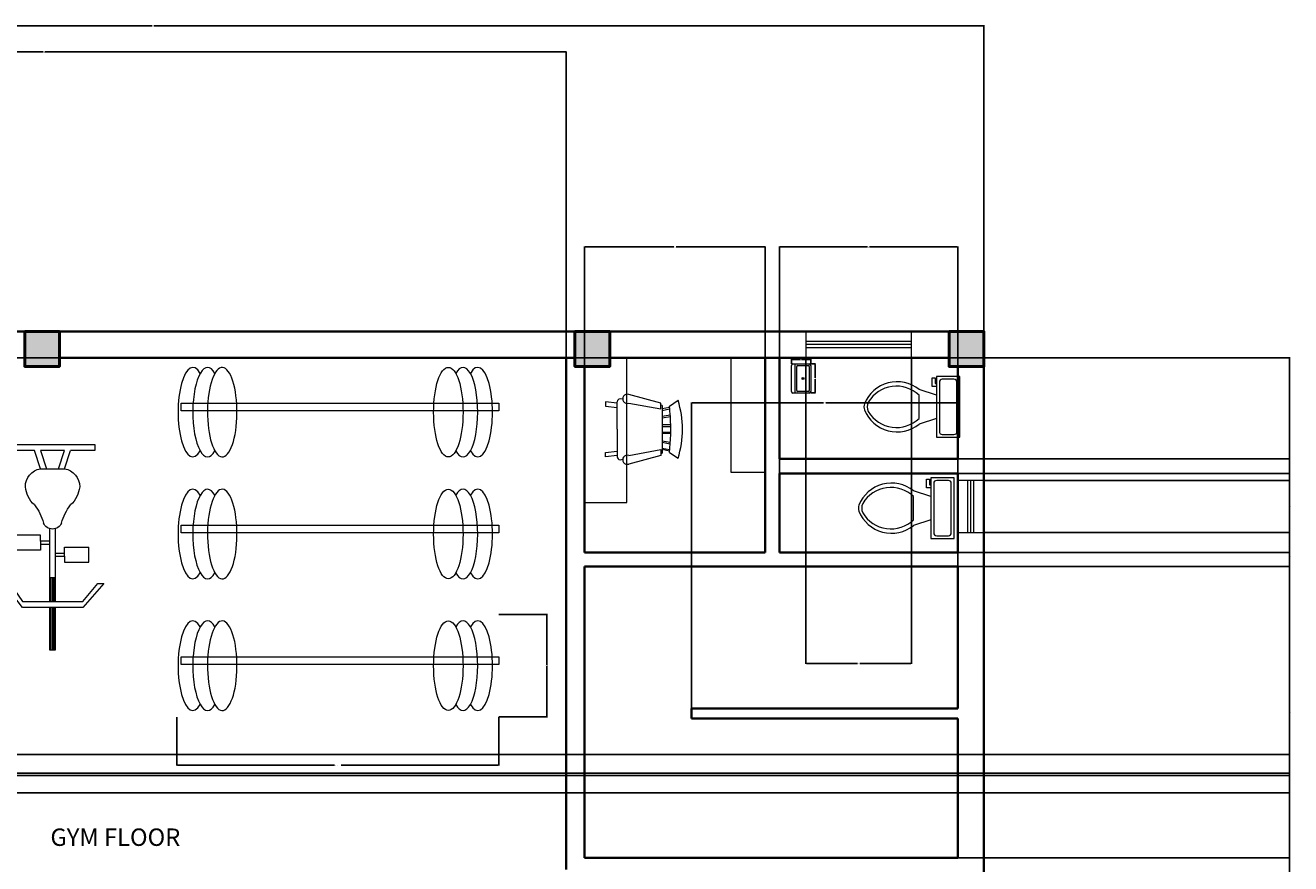
# Model space of a CAD drawing. Units: inches. Extents: x 369 to 4994, y 516 to 1297.
# Tile 9 of 9: x 2235 to 2672, y 855 to 1144. Entities that reach past the tile are written whole.
import ezdxf

# ---------------------------------------------------------------- set-up
doc = ezdxf.new("R2010")
doc.units = ezdxf.units.IN
doc.header["$MEASUREMENT"] = 0
for name, color, linetype, lineweight in [('A-ANNO-DIMS', 2, 'Continuous', 18), ('A-AREA-IDEN', 7, 'Continuous', 18), ('A-COLS', 7, 'Continuous', 50), ('A-EQPM', 9, 'Continuous', 18), ('A-FLOR-CASE', 8, 'Continuous', 18), ('A-FLOR-FIXT', 9, 'Continuous', 18), ('A-FURN', 8, 'Continuous', 18), ('A-GLAZ', 4, 'Continuous', 18), ('A-WALL', 7, 'Continuous', 35)]:
    doc.layers.add(name, color=color, linetype=linetype, lineweight=lineweight)
doc.layers.add('A-COLS-PATT', color=18, linetype='Continuous', lineweight=13, true_color=0x000000)
doc.styles.get("Standard").update_dxf_attribs({"font": 'arial.ttf'})
doc.dimstyles.get("Standard").update_dxf_attribs({"dimtxt": 0.18, "dimasz": 0.18, "dimexe": 0.18, "dimexo": 0.0625, "dimgap": 0.09, "dimtad": 0, "dimtih": 1, "dimtoh": 1, "dimdec": 4, "dimzin": 0, "dimdsep": 46, "dimtxsty": 'Standard', "dimcen": 0.09, "dimadec": 0, "dimazin": 0, "dimtfac": 1, "dimtdec": 4, "dimtofl": 0, "dimtmove": 0, "dimatfit": 3, "dimfxl": 1, "dimtolj": 1, "dimtzin": 0, "dimarcsym": 0})

# ---------------------------------------------------------------- blocks, each defined once
blk = doc.blocks.new('Sink-single - 30 in top')
blk.add_line((-15, -3.999996), (15, -3.999996))
for points in [[(-13.5, 0), (13.5, 0)], [(-15, -18.499996), (-15, -1.5)], [(-13.5, -17.499996), (-13.5, -6.499996)], [(-12.5, -5.499996), (12.5, -5.499996)], [(13.5, -6.499996), (13.5, -17.499996)], [(15, -1.5), (15, -18.499996)], [(13.5, -19.999996), (-13.5, -19.999996)], [(12.5, -18.499996), (-12.5, -18.499996)]]:
    blk.add_lwpolyline(points)
for radius in [1, 0.5]:
    blk.add_circle((0, -11.999996), radius)
for centre, radius, start, end in [((-13.5, -1.5), 1.5, 90, 180), ((-12.5, -6.499996), 1, 90, 180), ((12.5, -6.499996), 1, 0, 90), ((13.5, -1.5), 1.5, 0, 90), ((-13.5, -18.499996), 1.5, 180, 270), ((-12.5, -17.499996), 1, 180, 270), ((12.5, -17.499996), 1, 270, 0), ((13.5, -18.499996), 1.5, 270, 0)]:
    blk.add_arc(centre, radius, start, end)
blk = doc.blocks.new('Chair - Rocking')
for p, q in [((-8, -4.5), (-10, -1.5)), ((-4.5, -7), (-4.96674, -4.19951)), ((-4, -7), (-4.40532, -4.16272)), ((-1.5, -4.05012), (-1.5, -7)), ((-1, -7), (-1, -4.05012)), ((1, -7), (1, -4.04655)), ((1.5, -4.05012), (1.5, -7)), ((4, -7), (4.40187, -4.18694)), ((4.5, -7), (4.96761, -4.19437)), ((8, -4.5), (10, -1.5)), ((-9, -7.5), (-12, -18.49999)), ((-7, -7.5), (-9, -7.5)), ((-9, -18.49999), (-7, -7.5)), ((-8.23428, -6.99939), (-8.3093, -7.47958)), ((-8.23041, -7), (8.23915, -7)), ((-7.5, -4.5), (-7, -7)), ((-6.5, -7), (-7.02225, -4.43)), ((6.5, -7), (7, -4.4057)), ((7.5, -4.5), (7, -7)), ((7, -7.5), (9, -7.5)), ((9, -18.49999), (7, -7.5)), ((8.31071, -7.48854), (8.23449, -7.00073)), ((9, -7.5), (12, -18.49999)), ((-10.36644, -20.64523), (-10.5, -21.49999)), ((10.5, -21.49999), (10.3575, -20.58798)), ((-9, -22.49999), (-9.5, -26.49999)), ((0, -22.49999), (-9.5, -22.49999)), ((-8, -26.49999), (-7.5, -22.49999)), ((0, -22.49999), (9.5, -22.49999)), ((8, -26.49999), (7.5, -22.49999)), ((9, -22.49999), (9.5, -26.49999)), ((-9.5, -26.49999), (-8, -26.49999)), ((9.5, -26.49999), (8, -26.49999))]:
    blk.add_line(p, q)
for centre, radius, start, end in [((0, -34.08333), 34.08333, 72.93847, 107.0615), ((0, -68.25004), 64.25, 93.92211, 97.15267), ((0, -68.25004), 64.25, 82.84733, 93.92211), ((-10.5, -18.99999), 1.58114, 161.5651, 18.43495), ((-9.5, -21.49999), 1, 180, 270), ((10.5, -18.99999), 1.58114, 161.5651, 18.43495), ((9.5, -21.49999), 1, 270, 0)]:
    blk.add_arc(centre, radius, start, end)
blk = doc.blocks.new('Toilet - top')
for p, q in [((9.5, -6), (9.5, -2)), ((-10, -8.5), (-8, -8.5)), ((-10, -9.5), (-10, -8.5)), ((-8, -8.5), (-8, -8)), ((-7, -8), (-7, -9.5)), ((-4, -8), (-6, -14)), ((4, -8), (6, -14)), ((-7, -9.5), (-10, -9.5)), ((4, -14), (-4, -14))]:
    blk.add_line(p, q)
blk.add_lwpolyline([(10.5, -8), (10.5, 0), (-10.5, 0), (-10.5, -8)], close=True)
for points in [[(-9.5, -2), (-9.5, -6)], [(8.5, -1), (-8.5, -1)], [(-8.5, -7), (8.5, -7)]]:
    blk.add_lwpolyline(points)
for centre, radius, start, end in [((-8.62, -1.88), 0.884, 81.8699, 188.1301), ((8.62, -1.88), 0.884, 351.8699, 98.1301), ((-8.62, -6.12), 0.884, 171.8699, 278.1301), ((8.62, -6.12), 0.884, 261.8699, 8.1301), ((3.52, -21.58), 12.17, 141.4691, 247.9714), ((4.2, -21.82), 11.33, 136.3677, 238.9468), ((-3.52, -21.58), 12.17, 292.0284, 38.5307), ((-4.2, -21.82), 11.33, 301.053, 43.6321), ((0, -27.88), 4, 245.7318, 294.2682), ((0, -29), 4, 254.8605, 285.1395)]:
    blk.add_arc(centre, radius, start, end)
blk = doc.blocks.new('Exercise Bike')
for p, q in [((-0.75, 10), (-0.75, 17)), ((-0.75, 17), (0.25, 17)), ((-0.5, 17), (-0.5, 9.9929)), ((-0.25, 10), (-0.25, 17)), ((0, 17), (0, 9.9929)), ((0.25, 17), (0.25, 10)), ((-5.25, 10), (-8.25, 6)), ((-7.25, 6), (-5.25, 9)), ((-0.75, 10), (-5.25, 10)), ((-5.25, 9), (4.75, 9)), ((4.75, 10), (-0.75, 10)), ((-0.75, 5), (-0.75, 9)), ((-0.5, 8.9396), (-0.5, 5)), ((-0.25, 5), (-0.25, 9)), ((0, 8.9396), (0, 5)), ((0.25, 9), (0.25, 5)), ((8.25, 6), (4.75, 10)), ((4.75, 9), (7.25, 6)), ((-8.25, 6), (-7.25, 6)), ((-0.75, -3.0635), (-0.75, 5)), ((-0.75, 5), (0.25, 5)), ((0.25, 5), (0.25, -3.0635)), ((7.25, 6), (8.25, 6)), ((1.75, 2.5), (5.75, 2.5)), ((1.75, 1.5), (1.75, 2.5)), ((5.75, 2.5), (5.75, 0)), ((-6.25, -2), (-6.25, 0.5)), ((-2.25, 0.5), (-6.25, 0.5)), ((-2.25, -0.5), (-2.25, 0.5)), ((0.25, 1.5), (1.75, 1.5)), ((0.25, 1), (1.75, 1)), ((1.75, 1.5), (1.75, 0)), ((1.75, 0), (5.75, 0)), ((-2.25, -2), (-6.25, -2)), ((-2.25, -0.5), (-0.75, -0.5)), ((-2.25, -1), (-2.25, -0.5)), ((-2.25, -1), (-2.25, -2)), ((-0.75, -1), (-2.25, -1)), ((-2.25, -13), (-3.25, -16)), ((-2.25, -16), (-1.25, -13)), ((-2.25, -13), (1.75, -13)), ((0.75, -13), (1.75, -16)), ((1.75, -13), (2.75, -16)), ((-7.25, -16), (-7.25, -17)), ((-4.75, -16), (-7.25, -16)), ((-3.25, -16), (-4.75, -16)), ((1.75, -16), (-2.25, -16)), ((6.75, -16), (2.75, -16)), ((6.75, -17), (6.75, -16)), ((-7.25, -17), (6.75, -17))]:
    blk.add_line(p, q)
for centre, radius, start, end in [((-9.6692, -1.9154), 8.1889, 321.6175, 345.2525), ((-0.25, -4.625), 1.625, 22.61987, 157.3801), ((9.1691, -1.9154), 8.1889, 194.7476, 218.3825), ((0.1685, -10.5843), 4.9531, 133.6443, 173.2256), ((-0.6686, -10.5843), 4.9531, 6.774486, 46.35562), ((-1.7006, -10.0005), 3.0494, 179.9906, 259.6205), ((1.2006, -10.0005), 3.0494, 280.3795, 0.009389)]:
    blk.add_arc(centre, radius, start, end)
blk = doc.blocks.new('GYM-BARBELL')
blk.add_lwpolyline([(1.03, 18.49), (110.54, 18.49), (110.54, 15.84), (1.03, 15.84)], close=True)
for centre, start_param, end_param in [((5.08, 15.44), 5.759587, 9.948377), ((10.16, 15.44), 5.759587, 7.828079), ((15.23, 15.44), 1.544894, 7.828079), ((93.18, 15.44), 3.665191429188082, 9.948376736367669), ((98.25, 15.44), 3.665191, 6.806784), ((103.33, 15.44), 2.617994, 6.806784), ((10.16, 15.44), 7.828079, 9.948377), ((98.25, 15.44), 8.901179, 9.948377)]:
    blk.add_ellipse(centre, major_axis=(0, 15.44), ratio=0.328859, start_param=start_param, end_param=end_param)
blk = doc.blocks.new('*D29')
at = {"layer": 'A-ANNO-DIMS', "color": 0, "lineweight": -2, "transparency": 16777216}
for p, q in [((2506.3, 1027.62), (2507.92, 1027.62)), ((2507.74, 1027.44), (2507.74, 1022.8)), ((2507.74, 1017.79), (2507.74, 1022.43)), ((2506.3, 1017.61), (2507.92, 1017.61))]:
    blk.add_line(p, q, dxfattribs=at)
at = {"layer": 'A-ANNO-DIMS', "color": 0, "transparency": 16777216}
for points in [[(2507.71, 1027.44), (2507.77, 1027.44), (2507.74, 1027.62)], [(2507.71, 1017.79), (2507.77, 1017.79), (2507.74, 1017.61)]]:
    blk.add_solid(points, dxfattribs=at)
at = {"layer": 'Defpoints', "color": 0, "transparency": 16777216}
for p in [(2506.24, 1027.62), (2507.74, 1027.62), (2506.24, 1017.61)]:
    blk.add_point(p, dxfattribs=at)
at = {"layer": 'A-ANNO-DIMS', "color": 0, "transparency": 16777216, "insert": (2507.74, 1022.61), "char_height": 0.18, "attachment_point": 5}
blk.add_mtext('\\A1;SINK 10', dxfattribs=at)
blk = doc.blocks.new('*D30')
at = {"layer": 'A-ANNO-DIMS', "color": 0, "lineweight": -2, "transparency": 16777216}
for p, q in [((2499.56, 1027.69), (2499.56, 1029.31)), ((2499.74, 1029.13), (2502.75, 1029.13)), ((2506.06, 1029.13), (2503.04, 1029.13)), ((2506.24, 1027.69), (2506.24, 1029.31))]:
    blk.add_line(p, q, dxfattribs=at)
at = {"layer": 'A-ANNO-DIMS', "color": 0, "transparency": 16777216}
for points in [[(2499.74, 1029.16), (2499.74, 1029.1), (2499.56, 1029.13)], [(2506.06, 1029.16), (2506.06, 1029.1), (2506.24, 1029.13)]]:
    blk.add_solid(points, dxfattribs=at)
at = {"layer": 'Defpoints', "color": 0, "transparency": 16777216}
for p in [(2499.56, 1029.13), (2499.56, 1027.62), (2506.24, 1027.62)]:
    blk.add_point(p, dxfattribs=at)
at = {"layer": 'A-ANNO-DIMS', "color": 0, "transparency": 16777216, "insert": (2502.9, 1029.13), "char_height": 0.18, "attachment_point": 5}
blk.add_mtext('\\A1;7', dxfattribs=at)
blk = doc.blocks.new('*D35')
at = {"layer": 'A-ANNO-DIMS', "color": 0, "lineweight": -2, "transparency": 16777216}
for p, q in [((2287.71, 905.9), (2287.71, 889.14)), ((2398.64, 905.9), (2398.64, 889.14)), ((2287.89, 889.32), (2341.98, 889.32)), ((2398.46, 889.32), (2344.37, 889.32))]:
    blk.add_line(p, q, dxfattribs=at)
at = {"layer": 'A-ANNO-DIMS', "color": 0, "transparency": 16777216}
for points in [[(2287.89, 889.35), (2287.89, 889.29), (2287.71, 889.32)], [(2398.46, 889.35), (2398.46, 889.29), (2398.64, 889.32)]]:
    blk.add_solid(points, dxfattribs=at)
at = {"layer": 'Defpoints', "color": 0, "transparency": 16777216}
for p in [(2287.71, 905.96), (2398.64, 905.96), (2398.64, 889.32)]:
    blk.add_point(p, dxfattribs=at)
at = {"layer": 'A-ANNO-DIMS', "color": 0, "transparency": 16777216, "insert": (2343.18, 889.32), "char_height": 0.18, "attachment_point": 5}
blk.add_mtext('\\A1;BARBELL 111 TYP.', dxfattribs=at)
blk = doc.blocks.new('*D36')
at = {"layer": 'A-ANNO-DIMS', "color": 0, "lineweight": -2, "transparency": 16777216}
for p, q in [((2398.7, 941.23), (2415.46, 941.23)), ((2415.28, 941.05), (2415.28, 923.78)), ((2415.28, 906.14), (2415.28, 923.41)), ((2398.7, 905.96), (2415.46, 905.96))]:
    blk.add_line(p, q, dxfattribs=at)
at = {"layer": 'A-ANNO-DIMS', "color": 0, "transparency": 16777216}
for points in [[(2415.25, 941.05), (2415.31, 941.05), (2415.28, 941.23)], [(2415.25, 906.14), (2415.31, 906.14), (2415.28, 905.96)]]:
    blk.add_solid(points, dxfattribs=at)
at = {"layer": 'Defpoints', "color": 0, "transparency": 16777216}
for p in [(2398.64, 941.23), (2415.28, 941.23), (2398.64, 905.96)]:
    blk.add_point(p, dxfattribs=at)
at = {"layer": 'A-ANNO-DIMS', "color": 0, "transparency": 16777216, "insert": (2415.28, 923.6), "char_height": 0.18, "attachment_point": 5}
blk.add_mtext('\\A1;35 TYP.', dxfattribs=at)
blk = doc.blocks.new('*D46')
at = {"layer": 'A-ANNO-DIMS', "color": 0, "lineweight": -2, "transparency": 16777216}
for p, q in [((978.32, 1029.79), (2671.51, 1029.79)), ((2671.33, 1029.61), (2671.33, 957.97)), ((2671.33, 885.97), (2671.33, 957.61)), ((1038.32, 885.79), (2671.51, 885.79))]:
    blk.add_line(p, q, dxfattribs=at)
at = {"layer": 'A-ANNO-DIMS', "color": 0, "transparency": 16777216}
for points in [[(2671.3, 1029.61), (2671.36, 1029.61), (2671.33, 1029.79)], [(2671.3, 885.97), (2671.36, 885.97), (2671.33, 885.79)]]:
    blk.add_solid(points, dxfattribs=at)
at = {"layer": 'Defpoints', "color": 0, "transparency": 16777216}
for p in [(978.26, 1029.79), (2671.33, 1029.79), (1038.26, 885.79)]:
    blk.add_point(p, dxfattribs=at)
at = {"layer": 'A-ANNO-DIMS', "color": 0, "transparency": 16777216, "insert": (2671.33, 957.79), "char_height": 0.18, "attachment_point": 5}
blk.add_mtext('\\A1;144', dxfattribs=at)
blk = doc.blocks.new('*D47')
at = {"layer": 'A-ANNO-DIMS', "color": 0, "lineweight": -2, "transparency": 16777216}
for p, q in [((1038.32, 879.79), (2671.51, 879.79)), ((2671.33, 879.61), (2671.33, 837.52)), ((2671.33, 795.07), (2671.33, 837.16)), ((1035.32, 794.89), (2671.51, 794.89))]:
    blk.add_line(p, q, dxfattribs=at)
at = {"layer": 'A-ANNO-DIMS', "color": 0, "transparency": 16777216}
for points in [[(2671.3, 879.61), (2671.36, 879.61), (2671.33, 879.79)], [(2671.3, 795.07), (2671.36, 795.07), (2671.33, 794.89)]]:
    blk.add_solid(points, dxfattribs=at)
at = {"layer": 'Defpoints', "color": 0, "transparency": 16777216}
for p in [(1038.26, 879.79), (2671.33, 879.79), (1035.26, 794.89)]:
    blk.add_point(p, dxfattribs=at)
at = {"layer": 'A-ANNO-DIMS', "color": 0, "transparency": 16777216, "insert": (2671.33, 837.34), "char_height": 0.18, "attachment_point": 5}
blk.add_mtext('\\A1;84.9', dxfattribs=at)
blk = doc.blocks.new('*D79')
at = {"layer": 'A-ANNO-DIMS', "color": 0, "lineweight": -2, "transparency": 16777216}
for p, q in [((1769.44, 1029.79), (2671.51, 1029.79)), ((2671.33, 1029.61), (2671.33, 961.56)), ((2671.33, 893.15), (2671.33, 961.2)), ((1772.44, 892.97), (2671.51, 892.97))]:
    blk.add_line(p, q, dxfattribs=at)
at = {"layer": 'A-ANNO-DIMS', "color": 0, "transparency": 16777216}
for points in [[(2671.3, 1029.61), (2671.36, 1029.61), (2671.33, 1029.79)], [(2671.3, 893.15), (2671.36, 893.15), (2671.33, 892.97)]]:
    blk.add_solid(points, dxfattribs=at)
at = {"layer": 'Defpoints', "color": 0, "transparency": 16777216}
for p in [(1769.37, 1029.79), (2671.33, 1029.79), (1772.37, 892.97)]:
    blk.add_point(p, dxfattribs=at)
at = {"layer": 'A-ANNO-DIMS', "color": 0, "transparency": 16777216, "insert": (2671.33, 961.38), "char_height": 0.18, "attachment_point": 5}
blk.add_mtext('\\A1;136.82', dxfattribs=at)
blk = doc.blocks.new('*D80')
at = {"layer": 'A-ANNO-DIMS', "color": 0, "lineweight": -2, "transparency": 16777216}
for p, q in [((1772.44, 886.6), (2671.51, 886.6)), ((2671.33, 886.42), (2671.33, 847.38)), ((2671.33, 807.97), (2671.33, 847.01)), ((1772.44, 807.79), (2671.51, 807.79))]:
    blk.add_line(p, q, dxfattribs=at)
at = {"layer": 'A-ANNO-DIMS', "color": 0, "transparency": 16777216}
for points in [[(2671.3, 886.42), (2671.36, 886.42), (2671.33, 886.6)], [(2671.3, 807.97), (2671.36, 807.97), (2671.33, 807.79)]]:
    blk.add_solid(points, dxfattribs=at)
at = {"layer": 'Defpoints', "color": 0, "transparency": 16777216}
for p in [(1772.37, 886.6), (2671.33, 886.6), (1772.37, 807.79)]:
    blk.add_point(p, dxfattribs=at)
at = {"layer": 'A-ANNO-DIMS', "color": 0, "transparency": 16777216, "insert": (2671.33, 847.19), "char_height": 0.18, "attachment_point": 5}
blk.add_mtext('\\A1;78.81', dxfattribs=at)
blk = doc.blocks.new('*D97')
at = {"layer": 'A-ANNO-DIMS', "color": 0, "lineweight": -2, "transparency": 16777216}
for p, q in [((1992.93, 1038.85), (1992.93, 1144.37)), ((1993.11, 1144.19), (2279.14, 1144.19)), ((2565.75, 1144.19), (2279.72, 1144.19)), ((2565.93, 1038.85), (2565.93, 1144.37))]:
    blk.add_line(p, q, dxfattribs=at)
at = {"layer": 'A-ANNO-DIMS', "color": 0, "transparency": 16777216}
for points in [[(1993.11, 1144.22), (1993.11, 1144.16), (1992.93, 1144.19)], [(2565.75, 1144.22), (2565.75, 1144.16), (2565.93, 1144.19)]]:
    blk.add_solid(points, dxfattribs=at)
at = {"layer": 'Defpoints', "color": 0, "transparency": 16777216}
for p in [(2565.93, 1144.19), (1992.93, 1038.79), (2565.93, 1038.79)]:
    blk.add_point(p, dxfattribs=at)
at = {"layer": 'A-ANNO-DIMS', "color": 0, "transparency": 16777216, "insert": (2279.43, 1144.19), "char_height": 0.18, "attachment_point": 5}
blk.add_mtext('\\A1;573', dxfattribs=at)
blk = doc.blocks.new('*D99')
at = {"layer": 'A-ANNO-DIMS', "color": 0, "lineweight": -2, "transparency": 16777216}
for p, q in [((2061.93, 1029.85), (2061.93, 1135.37)), ((2062.11, 1135.19), (2241.64, 1135.19)), ((2421.75, 1135.19), (2242.22, 1135.19)), ((2421.93, 1029.85), (2421.93, 1135.37))]:
    blk.add_line(p, q, dxfattribs=at)
at = {"layer": 'A-ANNO-DIMS', "color": 0, "transparency": 16777216}
for points in [[(2062.11, 1135.22), (2062.11, 1135.16), (2061.93, 1135.19)], [(2421.75, 1135.22), (2421.75, 1135.16), (2421.93, 1135.19)]]:
    blk.add_solid(points, dxfattribs=at)
at = {"layer": 'Defpoints', "color": 0, "transparency": 16777216}
for p in [(2421.93, 1135.19), (2061.93, 1029.79), (2421.93, 1029.79)]:
    blk.add_point(p, dxfattribs=at)
at = {"layer": 'A-ANNO-DIMS', "color": 0, "transparency": 16777216, "insert": (2241.93, 1135.19), "char_height": 0.18, "attachment_point": 5}
blk.add_mtext('\\A1;360', dxfattribs=at)
blk = doc.blocks.new('*D100')
at = {"layer": 'A-ANNO-DIMS', "color": 0, "lineweight": -2, "transparency": 16777216}
for p, q in [((2428.28, 962.63), (2428.28, 1068.15)), ((2428.46, 1067.97), (2459.03, 1067.97)), ((2490.38, 1067.97), (2459.82, 1067.97)), ((2490.56, 962.63), (2490.56, 1068.15))]:
    blk.add_line(p, q, dxfattribs=at)
at = {"layer": 'A-ANNO-DIMS', "color": 0, "transparency": 16777216}
for points in [[(2428.46, 1068), (2428.46, 1067.94), (2428.28, 1067.97)], [(2490.38, 1068), (2490.38, 1067.94), (2490.56, 1067.97)]]:
    blk.add_solid(points, dxfattribs=at)
at = {"layer": 'Defpoints', "color": 0, "transparency": 16777216}
for p in [(2490.56, 1067.97), (2428.28, 962.57), (2490.56, 962.57)]:
    blk.add_point(p, dxfattribs=at)
at = {"layer": 'A-ANNO-DIMS', "color": 0, "transparency": 16777216, "insert": (2459.42, 1067.97), "char_height": 0.18, "attachment_point": 5}
blk.add_mtext('\\A1;62.28', dxfattribs=at)
blk = doc.blocks.new('*D101')
at = {"layer": 'A-ANNO-DIMS', "color": 0, "lineweight": -2, "transparency": 16777216}
for p, q in [((2495.43, 962.63), (2495.43, 1068.15)), ((2495.61, 1067.97), (2525.85, 1067.97)), ((2556.75, 1067.97), (2526.5, 1067.97)), ((2556.93, 962.63), (2556.93, 1068.15))]:
    blk.add_line(p, q, dxfattribs=at)
at = {"layer": 'A-ANNO-DIMS', "color": 0, "transparency": 16777216}
for points in [[(2495.61, 1068), (2495.61, 1067.94), (2495.43, 1067.97)], [(2556.75, 1068), (2556.75, 1067.94), (2556.93, 1067.97)]]:
    blk.add_solid(points, dxfattribs=at)
at = {"layer": 'Defpoints', "color": 0, "transparency": 16777216}
for p in [(2556.93, 1067.97), (2495.43, 962.57), (2556.93, 962.57)]:
    blk.add_point(p, dxfattribs=at)
at = {"layer": 'A-ANNO-DIMS', "color": 0, "transparency": 16777216, "insert": (2526.18, 1067.97), "char_height": 0.18, "attachment_point": 5}
blk.add_mtext('\\A1;61.5', dxfattribs=at)
blk = doc.blocks.new('*D102')
at = {"layer": 'A-ANNO-DIMS', "color": 0, "lineweight": -2, "transparency": 16777216}
for p, q in [((2553.99, 1029.79), (2671.51, 1029.79)), ((2671.33, 1029.61), (2671.33, 1012.51)), ((2671.33, 995.06), (2671.33, 1012.15)), ((2556.99, 994.88), (2671.51, 994.88))]:
    blk.add_line(p, q, dxfattribs=at)
at = {"layer": 'A-ANNO-DIMS', "color": 0, "transparency": 16777216}
for points in [[(2671.3, 1029.61), (2671.36, 1029.61), (2671.33, 1029.79)], [(2671.3, 995.06), (2671.36, 995.06), (2671.33, 994.88)]]:
    blk.add_solid(points, dxfattribs=at)
at = {"layer": 'Defpoints', "color": 0, "transparency": 16777216}
for p in [(2553.93, 1029.79), (2671.33, 1029.79), (2556.93, 994.88)]:
    blk.add_point(p, dxfattribs=at)
at = {"layer": 'A-ANNO-DIMS', "color": 0, "transparency": 16777216, "insert": (2671.33, 1012.33), "char_height": 0.18, "attachment_point": 5}
blk.add_mtext('\\A1;34.91', dxfattribs=at)
blk = doc.blocks.new('*D103')
at = {"layer": 'A-ANNO-DIMS', "color": 0, "lineweight": -2, "transparency": 16777216}
for p, q in [((2556.99, 989.85), (2671.51, 989.85)), ((2671.33, 989.67), (2671.33, 976.39)), ((2671.33, 962.75), (2671.33, 976.02)), ((2556.99, 962.57), (2671.51, 962.57))]:
    blk.add_line(p, q, dxfattribs=at)
at = {"layer": 'A-ANNO-DIMS', "color": 0, "transparency": 16777216}
for points in [[(2671.3, 989.67), (2671.36, 989.67), (2671.33, 989.85)], [(2671.3, 962.75), (2671.36, 962.75), (2671.33, 962.57)]]:
    blk.add_solid(points, dxfattribs=at)
at = {"layer": 'Defpoints', "color": 0, "transparency": 16777216}
for p in [(2556.93, 989.85), (2671.33, 989.85), (2556.93, 962.57)]:
    blk.add_point(p, dxfattribs=at)
at = {"layer": 'A-ANNO-DIMS', "color": 0, "transparency": 16777216, "insert": (2671.33, 976.21), "char_height": 0.18, "attachment_point": 5}
blk.add_mtext('\\A1;27.28', dxfattribs=at)
blk = doc.blocks.new('*D104')
at = {"layer": 'A-ANNO-DIMS', "color": 0, "lineweight": -2, "transparency": 16777216}
for p, q in [((2556.99, 957.85), (2671.51, 957.85)), ((2671.33, 957.67), (2671.33, 907.78)), ((2671.33, 857.52), (2671.33, 907.41)), ((2556.99, 857.34), (2671.51, 857.34))]:
    blk.add_line(p, q, dxfattribs=at)
at = {"layer": 'A-ANNO-DIMS', "color": 0, "transparency": 16777216}
for points in [[(2671.3, 957.67), (2671.36, 957.67), (2671.33, 957.85)], [(2671.3, 857.52), (2671.36, 857.52), (2671.33, 857.34)]]:
    blk.add_solid(points, dxfattribs=at)
at = {"layer": 'Defpoints', "color": 0, "transparency": 16777216}
for p in [(2556.93, 957.85), (2671.33, 957.85), (2556.93, 857.34)]:
    blk.add_point(p, dxfattribs=at)
at = {"layer": 'A-ANNO-DIMS', "color": 0, "transparency": 16777216, "insert": (2671.33, 907.6), "char_height": 0.18, "attachment_point": 5}
blk.add_mtext('\\A1;100.51', dxfattribs=at)
blk = doc.blocks.new('*D116')
at = {"layer": 'A-ANNO-DIMS', "color": 0, "lineweight": -2, "transparency": 16777216}
for p, q in [((2504.55, 1029.73), (2504.55, 924.21)), ((2540.94, 1029.73), (2540.94, 924.21)), ((2504.73, 924.39), (2522.35, 924.39)), ((2540.76, 924.39), (2523.14, 924.39))]:
    blk.add_line(p, q, dxfattribs=at)
at = {"layer": 'A-ANNO-DIMS', "color": 0, "transparency": 16777216}
for points in [[(2504.73, 924.42), (2504.73, 924.36), (2504.55, 924.39)], [(2540.76, 924.42), (2540.76, 924.36), (2540.94, 924.39)]]:
    blk.add_solid(points, dxfattribs=at)
at = {"layer": 'Defpoints', "color": 0, "transparency": 16777216}
for p in [(2504.55, 1029.79), (2540.94, 1029.79), (2504.55, 924.39)]:
    blk.add_point(p, dxfattribs=at)
at = {"layer": 'A-ANNO-DIMS', "color": 0, "transparency": 16777216, "insert": (2522.75, 924.39), "char_height": 0.18, "attachment_point": 5}
blk.add_mtext('\\A1;36.39', dxfattribs=at)
blk = doc.blocks.new('*D117')
at = {"layer": 'A-ANNO-DIMS', "color": 0, "lineweight": -2, "transparency": 16777216}
for p, q in [((2565.99, 987.42), (2671.51, 987.42)), ((2671.33, 987.24), (2671.33, 978.63)), ((2671.33, 969.66), (2671.33, 978.27)), ((2565.99, 969.48), (2671.51, 969.48))]:
    blk.add_line(p, q, dxfattribs=at)
at = {"layer": 'A-ANNO-DIMS', "color": 0, "transparency": 16777216}
for points in [[(2671.3, 987.24), (2671.36, 987.24), (2671.33, 987.42)], [(2671.3, 969.66), (2671.36, 969.66), (2671.33, 969.48)]]:
    blk.add_solid(points, dxfattribs=at)
at = {"layer": 'Defpoints', "color": 0, "transparency": 16777216}
for p in [(2565.93, 987.42), (2565.93, 969.48), (2671.33, 969.48)]:
    blk.add_point(p, dxfattribs=at)
at = {"layer": 'A-ANNO-DIMS', "color": 0, "transparency": 16777216, "insert": (2671.33, 978.45), "char_height": 0.18, "attachment_point": 5}
blk.add_mtext('\\A1;17.933', dxfattribs=at)
blk = doc.blocks.new('*D120')
at = {"layer": 'A-ANNO-DIMS', "color": 0, "lineweight": -2, "transparency": 16777216}
for p, q in [((2465.17, 908.87), (2465.17, 1014.39)), ((2465.35, 1014.21), (2510.65, 1014.21)), ((2556.75, 1014.21), (2511.44, 1014.21)), ((2556.93, 908.87), (2556.93, 1014.39))]:
    blk.add_line(p, q, dxfattribs=at)
at = {"layer": 'A-ANNO-DIMS', "color": 0, "transparency": 16777216}
for points in [[(2465.35, 1014.24), (2465.35, 1014.18), (2465.17, 1014.21)], [(2556.75, 1014.24), (2556.75, 1014.18), (2556.93, 1014.21)]]:
    blk.add_solid(points, dxfattribs=at)
at = {"layer": 'Defpoints', "color": 0, "transparency": 16777216}
for p in [(2556.93, 1014.21), (2465.17, 908.81), (2556.93, 908.81)]:
    blk.add_point(p, dxfattribs=at)
at = {"layer": 'A-ANNO-DIMS', "color": 0, "transparency": 16777216, "insert": (2511.05, 1014.21), "char_height": 0.18, "attachment_point": 5}
blk.add_mtext('\\A1;91.76', dxfattribs=at)

msp = doc.modelspace()

# ---------------------------------------------------------------- hatches: boundary and pattern name
at = {"layer": 'A-COLS-PATT'}
h = msp.add_hatch(color=256, dxfattribs=at)
h.dxf.hatch_style = 1
h.paths.add_polyline_path([(540.2581, 633.7894), (528.2581, 633.7894), (528.2581, 621.7894), (540.2581, 621.7894)])
h.paths.add_polyline_path([(726.2581, 633.7894), (714.2581, 633.7894), (714.2581, 621.7894), (726.2581, 621.7894)])
h.paths.add_polyline_path([(918.2581, 633.7894), (906.2581, 633.7894), (906.2581, 621.7894), (918.2581, 621.7894)])
h.paths.add_polyline_path([(1047.2581, 633.7894), (1035.2581, 633.7894), (1035.2581, 621.7894), (1047.2581, 621.7894)])
h.paths.add_polyline_path([(1047.2581, 798.6977), (1035.2581, 798.6977), (1035.2581, 786.6977), (1047.2581, 786.6977)])
h.paths.add_polyline_path([(918.2581, 795.7894), (906.2581, 795.7894), (906.2581, 783.7894), (918.2581, 783.7894)])
h.paths.add_polyline_path([(726.2581, 795.7894), (714.2581, 795.7894), (714.2581, 783.7894), (726.2581, 783.7894)])
h.paths.add_polyline_path([(1047.2581, 1038.7894), (1035.2581, 1038.7894), (1035.2581, 1026.7894), (1047.2581, 1026.7894)])
h.paths.add_polyline_path([(855.044, 1038.7894), (843.044, 1038.7894), (843.044, 1026.7894), (855.044, 1026.7894)])
h.paths.add_polyline_path([(728.5536, 1038.7894), (716.5536, 1038.7894), (716.5536, 1026.7894), (728.5536, 1026.7894)])
h.paths.add_polyline_path([(543.2581, 1038.7894), (531.2581, 1038.7894), (531.2581, 1026.7894), (543.2581, 1026.7894)])
h.paths.add_polyline_path([(543.2581, 792.9013), (531.2581, 792.9013), (531.2581, 780.9013), (543.2581, 780.9013), (543.2581, 783.7894)])
h.paths.add_polyline_path([(1274.3738, 633.7894), (1262.3738, 633.7894), (1262.3738, 621.7894), (1274.3738, 621.7894)])
h.paths.add_polyline_path([(1460.3738, 633.7894), (1448.3738, 633.7894), (1448.3738, 621.7894), (1460.3738, 621.7894)])
h.paths.add_polyline_path([(1652.3738, 633.7894), (1640.3738, 633.7894), (1640.3738, 621.7894), (1652.3738, 621.7894)])
h.paths.add_polyline_path([(1781.3738, 633.7894), (1769.3738, 633.7894), (1769.3738, 621.7894), (1781.3738, 621.7894)])
h.paths.add_polyline_path([(1781.3738, 1038.7894), (1769.3738, 1038.7894), (1769.3738, 1026.7894), (1781.3738, 1026.7894)])
h.paths.add_polyline_path([(1625.484, 1038.7894), (1613.484, 1038.7894), (1613.484, 1026.7894), (1615.6962, 1026.7894), (1625.484, 1026.7894)])
h.paths.add_polyline_path([(1462.6692, 1038.7894), (1450.6692, 1038.7894), (1450.6692, 1026.7894), (1462.6692, 1026.7894)])
h.paths.add_polyline_path([(1277.3738, 1038.7894), (1265.3738, 1038.7894), (1265.3738, 1026.7894), (1277.3738, 1026.7894)])
h.paths.add_polyline_path([(1460.3738, 807.7894), (1448.3738, 807.7894), (1448.3738, 795.7894), (1460.3738, 795.7894)])
h.paths.add_polyline_path([(1652.3738, 807.7894), (1640.3738, 807.7894), (1640.3738, 795.7894), (1652.3738, 795.7894)])
h.paths.add_polyline_path([(2244.9265, 633.7894), (2232.9265, 633.7894), (2232.9265, 621.7894), (2244.9265, 621.7894)])
h.paths.add_polyline_path([(2058.9265, 633.7894), (2046.9265, 633.7894), (2046.9265, 621.7894), (2058.9265, 621.7894)])
h.paths.add_polyline_path([(2436.9265, 633.7894), (2424.9265, 633.7894), (2424.9265, 621.7894), (2436.9265, 621.7894)])
h.paths.add_polyline_path([(2565.9265, 633.7894), (2553.9265, 633.7894), (2553.9265, 621.7894), (2565.9265, 621.7894)])
h.paths.add_polyline_path([(2565.9265, 798.6977), (2553.9265, 798.6977), (2553.9265, 786.6977), (2565.9265, 786.6977)])
h.paths.add_polyline_path([(2565.9265, 1038.7894), (2553.9265, 1038.7894), (2553.9265, 1026.7894), (2565.9265, 1026.7894)])
h.paths.add_polyline_path([(2436.9265, 1038.7894), (2424.9265, 1038.7894), (2424.9265, 1026.7894), (2436.9265, 1026.7894)])
h.paths.add_polyline_path([(2247.222, 1038.7894), (2235.222, 1038.7894), (2235.222, 1026.7894), (2247.222, 1026.7894)])
h.paths.add_polyline_path([(2061.9265, 1038.7894), (2049.9265, 1038.7894), (2049.9265, 1026.7894), (2061.9265, 1026.7894)])

# ---------------------------------------------------------------- linework, layer by layer
at = {"layer": 'A-COLS'}
for points in [[(2235.222, 1038.7894), (2247.222, 1038.7894), (2247.222, 1026.7894), (2235.222, 1026.7894)], [(2424.9265, 1038.7894), (2436.9265, 1038.7894), (2436.9265, 1026.7894), (2424.9265, 1026.7894)], [(2553.9265, 1038.7894), (2565.9265, 1038.7894), (2565.9265, 1026.7894), (2553.9265, 1026.7894)]]:
    msp.add_lwpolyline(points, close=True, dxfattribs=at)
at = {"layer": 'A-FLOR-CASE'}
msp.add_lwpolyline([(2428.2834, 1026.7894), (2428.2834, 979.9068), (2442.8807, 979.9068), (2442.8807, 1029.7894), (2436.9265, 1029.7894)], dxfattribs=at)
msp.add_lwpolyline([(2490.5616, 1029.7894), (2478.6323, 1029.7894), (2478.6323, 990.3401), (2490.5616, 990.3401)], close=True, dxfattribs=at)
at = {"layer": 'A-GLAZ'}
for p, q in [((2540.941, 1035.3655), (2504.5526, 1035.3655)), ((2540.941, 1034.2894), (2504.5526, 1034.2894)), ((2540.941, 1033.2133), (2504.5526, 1033.2133)), ((2560.3504, 969.4831), (2560.3504, 987.4162)), ((2561.4265, 969.4831), (2561.4265, 987.4162)), ((2562.5026, 969.4831), (2562.5026, 987.4162))]:
    msp.add_line(p, q, dxfattribs=at)
for points in [[(2504.5526, 1029.7894), (2540.941, 1029.7894), (2540.941, 1038.7894), (2504.5526, 1038.7894)], [(2556.9265, 969.4831), (2565.9265, 969.4831), (2565.9265, 987.4162), (2556.9265, 987.4162)]]:
    msp.add_lwpolyline(points, close=True, dxfattribs=at)
at = {"layer": 'A-WALL'}
for p, q in [((2556.9265, 1038.7894), (2049.9265, 1038.7894)), ((2361.7124, 1029.7894), (2247.222, 1029.7894)), ((2424.9265, 1029.7894), (2247.222, 1029.7894)), ((2424.9265, 1029.7894), (2373.7124, 1029.7894)), ((2421.9265, 908.8078), (2421.9265, 1029.7894)), ((2553.9265, 1029.7894), (2436.9265, 1029.7894)), ((2490.9265, 1029.7894), (2436.9265, 1029.7894)), ((2565.9265, 621.7894), (2565.9265, 1029.7894)), ((2428.2834, 962.568), (2428.2834, 1026.7894)), ((2556.9265, 994.8764), (2556.9265, 1026.7894)), ((2556.9265, 962.568), (2556.9265, 989.8457)), ((2428.2834, 857.3402), (2428.2834, 957.8515)), ((2556.9265, 908.8078), (2556.9265, 957.8515)), ((2421.9265, 908.8078), (2421.9265, 853.3402)), ((2556.9265, 908.8078), (2465.1694, 908.8078)), ((2465.1694, 905.3798), (2465.1694, 908.8078)), ((2556.9265, 905.3798), (2465.1694, 905.3798)), ((2556.9265, 857.3402), (2556.9265, 905.3798)), ((2556.9265, 857.3402), (2556.9265, 879.7894)), ((2556.9265, 857.3402), (2428.2834, 857.3402))]:
    msp.add_line(p, q, dxfattribs=at)
for points in [[(2495.4265, 994.8764), (2495.4265, 1029.7894), (2490.5616, 1029.7894), (2490.5616, 962.568)], [(2490.5616, 994.8764), (2490.5616, 989.8457)], [(2556.9265, 994.8764), (2495.4265, 994.8764)], [(2495.4265, 962.568), (2495.4265, 989.8457)], [(2495.4265, 989.8457), (2556.9265, 989.8457)], [(2490.5616, 962.568), (2428.2834, 962.568)], [(2556.9265, 962.568), (2495.4265, 962.568)], [(2428.2834, 957.8515), (2483.9184, 957.8515)], [(2428.2834, 957.8515), (2556.9265, 957.8515)]]:
    msp.add_lwpolyline(points, dxfattribs=at)

# ---------------------------------------------------------------- block references
at = {"layer": 'A-EQPM'}
for p in [(2288.107, 995.5724), (2288.107, 953.5332), (2288.107, 908.154)]:
    msp.add_blockref('GYM-BARBELL', p, dxfattribs=at)
at = {"layer": 'A-EQPM', "xscale": -2.080401215836593, "yscale": 2.080401215836593, "zscale": 2.080401215836593, "rotation": 180}
msp.add_blockref('Exercise Bike', (2245.3378, 964.4622), dxfattribs=at)
at = {"layer": 'A-FLOR-FIXT', "xscale": 0.3338934755196378, "yscale": 0.3338934755196378, "zscale": 0.3338934755196378, "rotation": 89.99999999999994}
msp.add_blockref('Sink-single - 30 in top', (2499.5577, 1022.6146), dxfattribs=at)
at = {"layer": 'A-FLOR-FIXT', "rotation": 269.9999999999999}
for p in [(2557.5878, 1012.8341), (2555.6766, 977.9149)]:
    msp.add_blockref('Toilet - top', p, dxfattribs=at)
at = {"layer": 'A-FURN', "rotation": 269.999999999998}
msp.add_blockref('Chair - Rocking', (2461.9903, 1005.1034), dxfattribs=at)

# ---------------------------------------------------------------- texts
at = {"layer": 'A-AREA-IDEN'}
msp.add_text(' GYM FLOOR ', height=6, dxfattribs=at).set_placement((2242.2655, 861.4773))

# ---------------------------------------------------------------- dimensions: what is measured, and where the dimension line sits
at = {"layer": 'A-ANNO-DIMS'}
for base, p1, p2, override, picture, middle in [((2565.9265, 1144.1894), (1992.9265, 1038.7894), (2565.9265, 1038.7894), {"dimdec": 0, "dimlfac": 1, "dimrnd": 0, "dimzin": 0, "dimdsep": 46, "dimlunit": 2}, '*D97', (2279.4265, 1144.1894)), ((2421.9265, 1135.1894), (2061.9265, 1029.7894), (2421.9265, 1029.7894), {"dimdec": 0, "dimlfac": 1, "dimrnd": 0, "dimzin": 0, "dimdsep": 46, "dimlunit": 2}, '*D99', (2241.9265, 1135.1894)), ((2490.5616, 1067.968), (2428.2834, 962.568), (2490.5616, 962.568), {"dimdec": 2, "dimlfac": 1, "dimrnd": 0, "dimzin": 0, "dimdsep": 46, "dimlunit": 2}, '*D100', (2459.4225, 1067.968)), ((2556.9265, 1067.968), (2495.4265, 962.568), (2556.9265, 962.568), {"dimdec": 1, "dimlfac": 1, "dimrnd": 0, "dimzin": 0, "dimdsep": 46, "dimlunit": 2}, '*D101', (2526.1765, 1067.968))]:
    dim = msp.add_linear_dim(base=base, p1=p1, p2=p2, dimstyle='Standard', override=override, dxfattribs=at)
    dim.commit()
    dim.dimension.update_dxf_attribs({"geometry": picture, "text_midpoint": middle})
for base, p1, p2, angle, override, picture, middle in [((2671.3265, 1029.7894), (1038.2581, 885.7894), (978.2581, 1029.7894), 90, {"dimdec": 0, "dimlfac": 1, "dimrnd": 0, "dimzin": 0, "dimdsep": 46, "dimlunit": 2}, '*D46', (2671.3265, 957.7894)), ((2671.3265, 1029.7894), (1772.3738, 892.9667), (1769.3738, 1029.7894), 90, {"dimdec": 2, "dimlfac": 1, "dimrnd": 0, "dimzin": 0, "dimdsep": 46, "dimlunit": 2}, '*D79', (2671.3265, 961.378)), ((2504.5526, 924.3894), (2540.941, 1029.7894), (2504.5526, 1029.7894), 180, {"dimdec": 2, "dimlfac": 1, "dimrnd": 0, "dimzin": 0, "dimdsep": 46, "dimlunit": 2}, '*D116', (2522.7468, 924.3894)), ((2671.3265, 1029.7894), (2556.9265, 994.8764), (2553.9265, 1029.7894), 90, {"dimdec": 2, "dimlfac": 1, "dimrnd": 0, "dimzin": 0, "dimdsep": 46, "dimlunit": 2}, '*D102', (2671.3265, 1012.3329)), ((2499.5577, 1029.1256), (2506.2356, 1027.623), (2499.5577, 1027.623), 180, {"dimdec": 0, "dimlfac": 1, "dimrnd": 0, "dimzin": 0, "dimdsep": 46, "dimlunit": 2}, '*D30', (2502.8966, 1029.1256)), ((2556.9265, 1014.2078), (2465.1694, 908.8078), (2556.9265, 908.8078), 0, {"dimdec": 2, "dimlfac": 1, "dimrnd": 0, "dimzin": 0, "dimdsep": 46, "dimlunit": 2}, '*D120', (2511.048, 1014.2078)), ((2671.3265, 989.8457), (2556.9265, 962.568), (2556.9265, 989.8457), 90, {"dimdec": 2, "dimlfac": 1, "dimrnd": 0, "dimzin": 0, "dimdsep": 46, "dimlunit": 2}, '*D103', (2671.3265, 976.2069)), ((2671.3265, 969.4831), (2565.9265, 987.4162), (2565.9265, 969.4831), 270, {"dimdec": 3, "dimlfac": 1, "dimrnd": 0, "dimzin": 0, "dimdsep": 46, "dimlunit": 2}, '*D117', (2671.3265, 978.4497)), ((2671.3265, 957.8515), (2556.9265, 857.3402), (2556.9265, 957.8515), 90, {"dimdec": 2, "dimlfac": 1, "dimrnd": 0, "dimzin": 0, "dimdsep": 46, "dimlunit": 2}, '*D104', (2671.3265, 907.5958)), ((2671.3265, 886.5988), (1772.3738, 807.7894), (1772.3738, 886.5988), 90, {"dimdec": 2, "dimlfac": 1, "dimrnd": 0, "dimzin": 0, "dimdsep": 46, "dimlunit": 2}, '*D80', (2671.3265, 847.1941)), ((2671.3265, 879.7894), (1035.2581, 794.8925), (1038.2581, 879.7894), 90, {"dimdec": 1, "dimlfac": 1, "dimrnd": 0, "dimzin": 0, "dimdsep": 46, "dimlunit": 2}, '*D47', (2671.3265, 837.3409))]:
    dim = msp.add_linear_dim(base=base, p1=p1, p2=p2, angle=angle, dimstyle='Standard', override=override, dxfattribs=at)
    dim.commit()
    dim.dimension.update_dxf_attribs({"geometry": picture, "text_midpoint": middle})
for base, p1, p2, text, picture, middle in [((2507.7381, 1027.623), (2506.2356, 1017.6062), (2506.2356, 1027.623), 'SINK <>', '*D29', (2507.7381, 1022.6146)), ((2415.282, 941.2342), (2398.6423, 905.9595), (2398.6423, 941.2342), '<> TYP.', '*D36', (2415.282, 923.5969))]:
    dim = msp.add_linear_dim(base=base, p1=p1, p2=p2, angle=90, text=text, dimstyle='Standard', override={"dimdec": 0, "dimlfac": 1, "dimrnd": 0, "dimzin": 0, "dimdsep": 46, "dimlunit": 2}, dxfattribs=at)
    dim.commit()
    dim.dimension.update_dxf_attribs({"geometry": picture, "text_midpoint": middle})
dim = msp.add_linear_dim(base=(2398.6423, 889.3198), p1=(2287.7112, 905.9595), p2=(2398.6423, 905.9595), text='BARBELL <> TYP.', dimstyle='Standard', override={"dimdec": 0, "dimlfac": 1, "dimrnd": 0, "dimzin": 0, "dimdsep": 46, "dimlunit": 2}, dxfattribs=at)
dim.commit()
dim.dimension.update_dxf_attribs({"geometry": '*D35', "text_midpoint": (2343.1767, 889.3198)})

doc.saveas('drawing.dxf')
